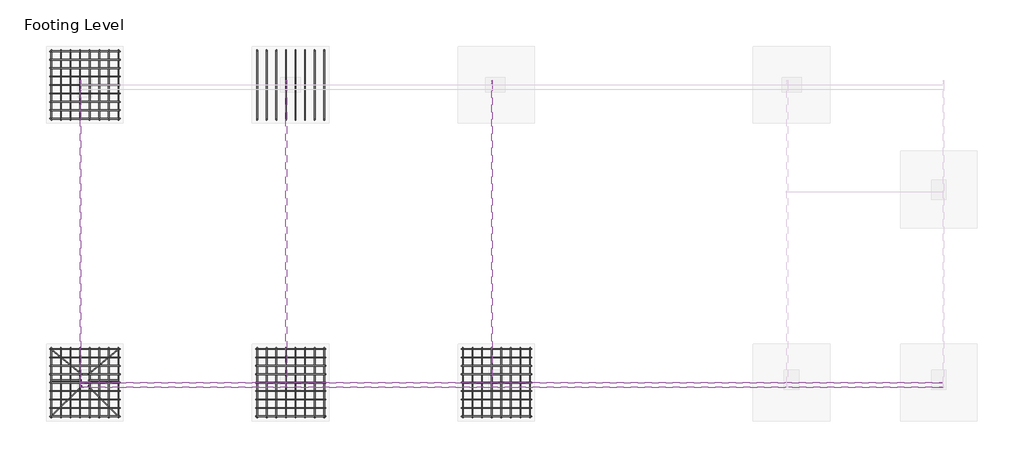
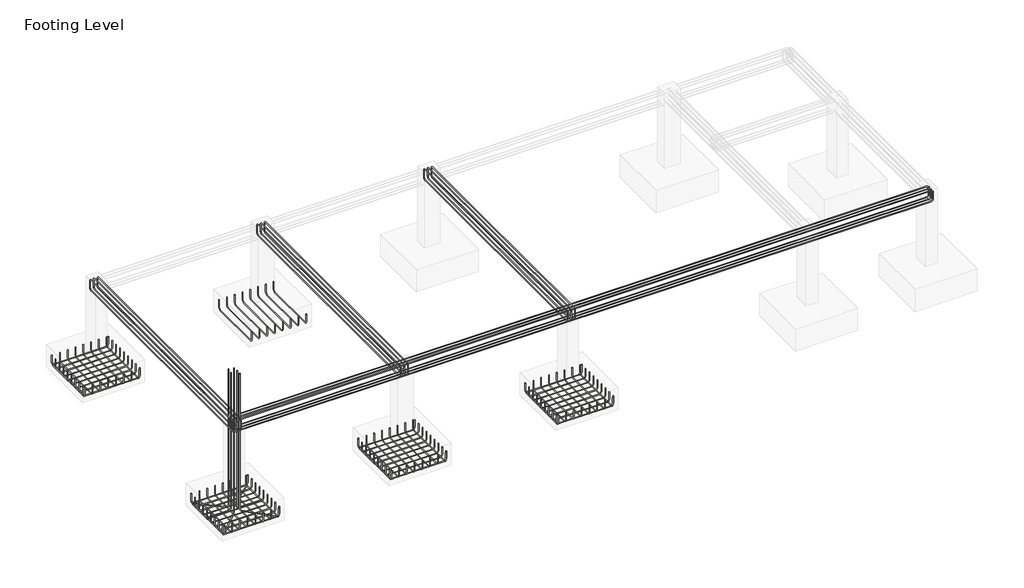
# One storey, part 2 of 3: 23 reinforcing bars.
"""IFC4 building model written with IfcOpenShell, lengths in millimetres."""

from ifc_helpers import new_model, si_unit, point, frame, origin, place, context, project, spatial, polyline, circle_curve, trimmed, segment, composite_curve, source, transform, mapped, element, save
from ifc_brep_helpers import swept_disk

model = new_model("IFC4")

# Units and contexts
model_context = context("Model", 3, world=origin())
ifc_project = project(units=[si_unit("LENGTHUNIT", "METRE", prefix="MILLI")], contexts=[model_context])

# Site, building, storey
site = spatial("IfcSite", under=ifc_project)
building = spatial("IfcBuilding", under=site)
storey = spatial("IfcBuildingStorey", under=building, Name="Footing Level", Elevation=-1524.0)

# Reinforcing bars
placement = place(None, origin())
reinforcing_bar_shape = source(origin(), model_context, "Body", "SolidModel", [
    swept_disk(composite_curve([segment(polyline([(-8741.5465807, -243.2665369, -1724.0), (-8741.5465807, -243.2665369, -1872.0)]), True, "CONTINUOUS"), segment(trimmed(circle_curve(frame((-8741.5465807, -197.2665369, -1872.0), z_axis=(1.0, 0.0, 0.0), x_axis=(0.0, -46.0, 0.0)), 46.0), [point((-8741.5465807, -243.2665369, -1872.0))], [point((-8741.5465807, -197.2665369, -1918.0))], True, "CARTESIAN"), True, "CONTINUOUS"), segment(polyline([(-8741.5465807, -197.2665369, -1918.0), (-8741.5465807, 798.7334631, -1918.0)]), True, "CONTINUOUS"), segment(trimmed(circle_curve(frame((-8741.5465807, 798.7334631, -1872.0), z_axis=(1.0, 0.0, 0.0), x_axis=(0.0, 0.0, -46.0)), 46.0), [point((-8741.5465807, 798.7334631, -1918.0))], [point((-8741.5465807, 844.7334631, -1872.0))], True, "CARTESIAN"), True, "CONTINUOUS"), segment(polyline([(-8741.5465807, 844.7334631, -1872.0), (-8741.5465807, 844.7334631, -1724.0)]), True, "CONTINUOUS")], self_intersect=False), 6.0),
])
element("IfcReinforcingBar", 1, at=placement, inside=storey, context=model_context, shape_type="MappedRepresentation", body=[
    mapped(reinforcing_bar_shape, transform((0.0, 0.0, 0.0), x_axis=(1.0, 0.0, 0.0), y_axis=(0.0, 1.0, 0.0), z_axis=(0.0, 0.0, 1.0))),
    mapped(reinforcing_bar_shape, transform((-149.7374868, 0.0, 0.0), x_axis=(1.0, 0.0, 0.0), y_axis=(0.0, 1.0, 0.0), z_axis=(0.0, 0.0, 1.0))),
    mapped(reinforcing_bar_shape, transform((-299.4749737, 0.0, 0.0), x_axis=(1.0, 0.0, 0.0), y_axis=(0.0, 1.0, 0.0), z_axis=(0.0, 0.0, 1.0))),
    mapped(reinforcing_bar_shape, transform((-449.2124605, 0.0, 0.0), x_axis=(1.0, 0.0, 0.0), y_axis=(0.0, 1.0, 0.0), z_axis=(0.0, 0.0, 1.0))),
    mapped(reinforcing_bar_shape, transform((-598.9499474, 0.0, 0.0), x_axis=(1.0, 0.0, 0.0), y_axis=(0.0, 1.0, 0.0), z_axis=(0.0, 0.0, 1.0))),
    mapped(reinforcing_bar_shape, transform((-748.6874342, 0.0, 0.0), x_axis=(1.0, 0.0, 0.0), y_axis=(0.0, 1.0, 0.0), z_axis=(0.0, 0.0, 1.0))),
    mapped(reinforcing_bar_shape, transform((-898.424921, 0.0, 0.0), x_axis=(1.0, 0.0, 0.0), y_axis=(0.0, 1.0, 0.0), z_axis=(0.0, 0.0, 1.0))),
    mapped(reinforcing_bar_shape, transform((-1048.1624079, 0.0, 0.0), x_axis=(1.0, 0.0, 0.0), y_axis=(0.0, 1.0, 0.0), z_axis=(0.0, 0.0, 1.0))),
])
reinforcing_bar_2_shape = source(origin(), model_context, "Body", "SolidModel", [
    swept_disk(composite_curve([segment(polyline([(-9808.6117524, -224.7796689, -1711.15), (-9808.6117524, -224.7796689, -1859.15)]), True, "CONTINUOUS"), segment(trimmed(circle_curve(frame((-9762.6117524, -224.7796689, -1859.15), z_axis=(0.0, -1.0, 0.0), x_axis=(-46.0, 0.0, 0.0)), 46.0), [point((-9808.6117524, -224.7796689, -1859.15))], [point((-9762.6117524, -224.7796689, -1905.15))], True, "CARTESIAN"), True, "CONTINUOUS"), segment(polyline([(-9762.6117524, -224.7796689, -1905.15), (-8766.6117524, -224.7796689, -1905.15)]), True, "CONTINUOUS"), segment(trimmed(circle_curve(frame((-8766.6117524, -224.7796689, -1859.15), z_axis=(0.0, -1.0, 0.0), x_axis=(0.0, 0.0, -46.0)), 46.0), [point((-8766.6117524, -224.7796689, -1905.15))], [point((-8720.6117524, -224.7796689, -1859.15))], True, "CARTESIAN"), True, "CONTINUOUS"), segment(polyline([(-8720.6117524, -224.7796689, -1859.15), (-8720.6117524, -224.7796689, -1711.15)]), True, "CONTINUOUS")], self_intersect=False), 6.0),
])
element("IfcReinforcingBar", 2, at=placement, inside=storey, context=model_context, shape_type="MappedRepresentation", body=[
    mapped(reinforcing_bar_2_shape, transform((0.0, 0.0, 0.0), x_axis=(1.0, 0.0, 0.0), y_axis=(0.0, 1.0, 0.0), z_axis=(0.0, 0.0, 1.0))),
    mapped(reinforcing_bar_2_shape, transform((0.0, 131.3537501, 0.0), x_axis=(1.0, 0.0, 0.0), y_axis=(0.0, 1.0, 0.0), z_axis=(0.0, 0.0, 1.0))),
    mapped(reinforcing_bar_2_shape, transform((0.0, 262.7075003, 0.0), x_axis=(1.0, 0.0, 0.0), y_axis=(0.0, 1.0, 0.0), z_axis=(0.0, 0.0, 1.0))),
    mapped(reinforcing_bar_2_shape, transform((0.0, 394.0612504, 0.0), x_axis=(1.0, 0.0, 0.0), y_axis=(0.0, 1.0, 0.0), z_axis=(0.0, 0.0, 1.0))),
    mapped(reinforcing_bar_2_shape, transform((0.0, 525.4150006, 0.0), x_axis=(1.0, 0.0, 0.0), y_axis=(0.0, 1.0, 0.0), z_axis=(0.0, 0.0, 1.0))),
    mapped(reinforcing_bar_2_shape, transform((0.0, 656.7687507, 0.0), x_axis=(1.0, 0.0, 0.0), y_axis=(0.0, 1.0, 0.0), z_axis=(0.0, 0.0, 1.0))),
    mapped(reinforcing_bar_2_shape, transform((0.0, 788.1225008, 0.0), x_axis=(1.0, 0.0, 0.0), y_axis=(0.0, 1.0, 0.0), z_axis=(0.0, 0.0, 1.0))),
    mapped(reinforcing_bar_2_shape, transform((0.0, 919.476251, 0.0), x_axis=(1.0, 0.0, 0.0), y_axis=(0.0, 1.0, 0.0), z_axis=(0.0, 0.0, 1.0))),
    mapped(reinforcing_bar_2_shape, transform((0.0, 1050.8300011, 0.0), x_axis=(1.0, 0.0, 0.0), y_axis=(0.0, 1.0, 0.0), z_axis=(0.0, 0.0, 1.0))),
])
reinforcing_bar_3_shape = source(origin(), model_context, "Body", "SolidModel", [
    swept_disk(composite_curve([segment(polyline([(-5528.4465807, -243.2665369, -1724.0), (-5528.4465807, -243.2665369, -1872.0)]), True, "CONTINUOUS"), segment(trimmed(circle_curve(frame((-5528.4465807, -197.2665369, -1872.0), z_axis=(1.0, 0.0, 0.0), x_axis=(0.0, -46.0, 0.0)), 46.0), [point((-5528.4465807, -243.2665369, -1872.0))], [point((-5528.4465807, -197.2665369, -1918.0))], True, "CARTESIAN"), True, "CONTINUOUS"), segment(polyline([(-5528.4465807, -197.2665369, -1918.0), (-5528.4465807, 798.7334631, -1918.0)]), True, "CONTINUOUS"), segment(trimmed(circle_curve(frame((-5528.4465807, 798.7334631, -1872.0), z_axis=(1.0, 0.0, 0.0), x_axis=(0.0, 0.0, -46.0)), 46.0), [point((-5528.4465807, 798.7334631, -1918.0))], [point((-5528.4465807, 844.7334631, -1872.0))], True, "CARTESIAN"), True, "CONTINUOUS"), segment(polyline([(-5528.4465807, 844.7334631, -1872.0), (-5528.4465807, 844.7334631, -1724.0)]), True, "CONTINUOUS")], self_intersect=False), 6.0),
])
element("IfcReinforcingBar", 3, at=placement, inside=storey, context=model_context, shape_type="MappedRepresentation", body=[
    mapped(reinforcing_bar_3_shape, transform((0.0, 0.0, 0.0), x_axis=(1.0, 0.0, 0.0), y_axis=(0.0, 1.0, 0.0), z_axis=(0.0, 0.0, 1.0))),
    mapped(reinforcing_bar_3_shape, transform((-149.7374868, 0.0, 0.0), x_axis=(1.0, 0.0, 0.0), y_axis=(0.0, 1.0, 0.0), z_axis=(0.0, 0.0, 1.0))),
    mapped(reinforcing_bar_3_shape, transform((-299.4749737, 0.0, 0.0), x_axis=(1.0, 0.0, 0.0), y_axis=(0.0, 1.0, 0.0), z_axis=(0.0, 0.0, 1.0))),
    mapped(reinforcing_bar_3_shape, transform((-449.2124605, 0.0, 0.0), x_axis=(1.0, 0.0, 0.0), y_axis=(0.0, 1.0, 0.0), z_axis=(0.0, 0.0, 1.0))),
    mapped(reinforcing_bar_3_shape, transform((-598.9499474, 0.0, 0.0), x_axis=(1.0, 0.0, 0.0), y_axis=(0.0, 1.0, 0.0), z_axis=(0.0, 0.0, 1.0))),
    mapped(reinforcing_bar_3_shape, transform((-748.6874342, 0.0, 0.0), x_axis=(1.0, 0.0, 0.0), y_axis=(0.0, 1.0, 0.0), z_axis=(0.0, 0.0, 1.0))),
    mapped(reinforcing_bar_3_shape, transform((-898.424921, 0.0, 0.0), x_axis=(1.0, 0.0, 0.0), y_axis=(0.0, 1.0, 0.0), z_axis=(0.0, 0.0, 1.0))),
    mapped(reinforcing_bar_3_shape, transform((-1048.1624079, 0.0, 0.0), x_axis=(1.0, 0.0, 0.0), y_axis=(0.0, 1.0, 0.0), z_axis=(0.0, 0.0, 1.0))),
])
reinforcing_bar_4_shape = source(origin(), model_context, "Body", "SolidModel", [
    swept_disk(composite_curve([segment(polyline([(-6595.5117524, -224.7796689, -1711.15), (-6595.5117524, -224.7796689, -1859.15)]), True, "CONTINUOUS"), segment(trimmed(circle_curve(frame((-6549.5117524, -224.7796689, -1859.15), z_axis=(0.0, -1.0, 0.0), x_axis=(-46.0, 0.0, 0.0)), 46.0), [point((-6595.5117524, -224.7796689, -1859.15))], [point((-6549.5117524, -224.7796689, -1905.15))], True, "CARTESIAN"), True, "CONTINUOUS"), segment(polyline([(-6549.5117524, -224.7796689, -1905.15), (-5553.5117524, -224.7796689, -1905.15)]), True, "CONTINUOUS"), segment(trimmed(circle_curve(frame((-5553.5117524, -224.7796689, -1859.15), z_axis=(0.0, -1.0, 0.0), x_axis=(0.0, 0.0, -46.0)), 46.0), [point((-5553.5117524, -224.7796689, -1905.15))], [point((-5507.5117524, -224.7796689, -1859.15))], True, "CARTESIAN"), True, "CONTINUOUS"), segment(polyline([(-5507.5117524, -224.7796689, -1859.15), (-5507.5117524, -224.7796689, -1711.15)]), True, "CONTINUOUS")], self_intersect=False), 6.0),
])
element("IfcReinforcingBar", 4, at=placement, inside=storey, context=model_context, shape_type="MappedRepresentation", body=[
    mapped(reinforcing_bar_4_shape, transform((0.0, 0.0, 0.0), x_axis=(1.0, 0.0, 0.0), y_axis=(0.0, 1.0, 0.0), z_axis=(0.0, 0.0, 1.0))),
    mapped(reinforcing_bar_4_shape, transform((0.0, 131.3537501, 0.0), x_axis=(1.0, 0.0, 0.0), y_axis=(0.0, 1.0, 0.0), z_axis=(0.0, 0.0, 1.0))),
    mapped(reinforcing_bar_4_shape, transform((0.0, 262.7075003, 0.0), x_axis=(1.0, 0.0, 0.0), y_axis=(0.0, 1.0, 0.0), z_axis=(0.0, 0.0, 1.0))),
    mapped(reinforcing_bar_4_shape, transform((0.0, 394.0612504, 0.0), x_axis=(1.0, 0.0, 0.0), y_axis=(0.0, 1.0, 0.0), z_axis=(0.0, 0.0, 1.0))),
    mapped(reinforcing_bar_4_shape, transform((0.0, 525.4150006, 0.0), x_axis=(1.0, 0.0, 0.0), y_axis=(0.0, 1.0, 0.0), z_axis=(0.0, 0.0, 1.0))),
    mapped(reinforcing_bar_4_shape, transform((0.0, 656.7687507, 0.0), x_axis=(1.0, 0.0, 0.0), y_axis=(0.0, 1.0, 0.0), z_axis=(0.0, 0.0, 1.0))),
    mapped(reinforcing_bar_4_shape, transform((0.0, 788.1225008, 0.0), x_axis=(1.0, 0.0, 0.0), y_axis=(0.0, 1.0, 0.0), z_axis=(0.0, 0.0, 1.0))),
    mapped(reinforcing_bar_4_shape, transform((0.0, 919.476251, 0.0), x_axis=(1.0, 0.0, 0.0), y_axis=(0.0, 1.0, 0.0), z_axis=(0.0, 0.0, 1.0))),
    mapped(reinforcing_bar_4_shape, transform((0.0, 1050.8300011, 0.0), x_axis=(1.0, 0.0, 0.0), y_axis=(0.0, 1.0, 0.0), z_axis=(0.0, 0.0, 1.0))),
])
reinforcing_bar_5_shape = source(origin(), model_context, "Body", "SolidModel", [
    swept_disk(composite_curve([segment(polyline([(-2315.3465807, -243.2665369, -1724.0), (-2315.3465807, -243.2665369, -1872.0)]), True, "CONTINUOUS"), segment(trimmed(circle_curve(frame((-2315.3465807, -197.2665369, -1872.0), z_axis=(1.0, 0.0, 0.0), x_axis=(0.0, -46.0, 0.0)), 46.0), [point((-2315.3465807, -243.2665369, -1872.0))], [point((-2315.3465807, -197.2665369, -1918.0))], True, "CARTESIAN"), True, "CONTINUOUS"), segment(polyline([(-2315.3465807, -197.2665369, -1918.0), (-2315.3465807, 798.7334631, -1918.0)]), True, "CONTINUOUS"), segment(trimmed(circle_curve(frame((-2315.3465807, 798.7334631, -1872.0), z_axis=(1.0, 0.0, 0.0), x_axis=(0.0, 0.0, -46.0)), 46.0), [point((-2315.3465807, 798.7334631, -1918.0))], [point((-2315.3465807, 844.7334631, -1872.0))], True, "CARTESIAN"), True, "CONTINUOUS"), segment(polyline([(-2315.3465807, 844.7334631, -1872.0), (-2315.3465807, 844.7334631, -1724.0)]), True, "CONTINUOUS")], self_intersect=False), 6.0),
])
element("IfcReinforcingBar", 5, at=placement, inside=storey, context=model_context, shape_type="MappedRepresentation", body=[
    mapped(reinforcing_bar_5_shape, transform((0.0, 0.0, 0.0), x_axis=(1.0, 0.0, 0.0), y_axis=(0.0, 1.0, 0.0), z_axis=(0.0, 0.0, 1.0))),
    mapped(reinforcing_bar_5_shape, transform((-149.7374868, 0.0, 0.0), x_axis=(1.0, 0.0, 0.0), y_axis=(0.0, 1.0, 0.0), z_axis=(0.0, 0.0, 1.0))),
    mapped(reinforcing_bar_5_shape, transform((-299.4749737, 0.0, 0.0), x_axis=(1.0, 0.0, 0.0), y_axis=(0.0, 1.0, 0.0), z_axis=(0.0, 0.0, 1.0))),
    mapped(reinforcing_bar_5_shape, transform((-449.2124605, 0.0, 0.0), x_axis=(1.0, 0.0, 0.0), y_axis=(0.0, 1.0, 0.0), z_axis=(0.0, 0.0, 1.0))),
    mapped(reinforcing_bar_5_shape, transform((-598.9499474, 0.0, 0.0), x_axis=(1.0, 0.0, 0.0), y_axis=(0.0, 1.0, 0.0), z_axis=(0.0, 0.0, 1.0))),
    mapped(reinforcing_bar_5_shape, transform((-748.6874342, 0.0, 0.0), x_axis=(1.0, 0.0, 0.0), y_axis=(0.0, 1.0, 0.0), z_axis=(0.0, 0.0, 1.0))),
    mapped(reinforcing_bar_5_shape, transform((-898.424921, 0.0, 0.0), x_axis=(1.0, 0.0, 0.0), y_axis=(0.0, 1.0, 0.0), z_axis=(0.0, 0.0, 1.0))),
    mapped(reinforcing_bar_5_shape, transform((-1048.1624079, 0.0, 0.0), x_axis=(1.0, 0.0, 0.0), y_axis=(0.0, 1.0, 0.0), z_axis=(0.0, 0.0, 1.0))),
])
reinforcing_bar_6_shape = source(origin(), model_context, "Body", "SolidModel", [
    swept_disk(composite_curve([segment(polyline([(-3382.4117524, -224.7796689, -1711.15), (-3382.4117524, -224.7796689, -1859.15)]), True, "CONTINUOUS"), segment(trimmed(circle_curve(frame((-3336.4117524, -224.7796689, -1859.15), z_axis=(0.0, -1.0, 0.0), x_axis=(-46.0, 0.0, 0.0)), 46.0), [point((-3382.4117524, -224.7796689, -1859.15))], [point((-3336.4117524, -224.7796689, -1905.15))], True, "CARTESIAN"), True, "CONTINUOUS"), segment(polyline([(-3336.4117524, -224.7796689, -1905.15), (-2340.4117524, -224.7796689, -1905.15)]), True, "CONTINUOUS"), segment(trimmed(circle_curve(frame((-2340.4117524, -224.7796689, -1859.15), z_axis=(0.0, -1.0, 0.0), x_axis=(0.0, 0.0, -46.0)), 46.0), [point((-2340.4117524, -224.7796689, -1905.15))], [point((-2294.4117524, -224.7796689, -1859.15))], True, "CARTESIAN"), True, "CONTINUOUS"), segment(polyline([(-2294.4117524, -224.7796689, -1859.15), (-2294.4117524, -224.7796689, -1711.15)]), True, "CONTINUOUS")], self_intersect=False), 6.0),
])
element("IfcReinforcingBar", 6, at=placement, inside=storey, context=model_context, shape_type="MappedRepresentation", body=[
    mapped(reinforcing_bar_6_shape, transform((0.0, 0.0, 0.0), x_axis=(1.0, 0.0, 0.0), y_axis=(0.0, 1.0, 0.0), z_axis=(0.0, 0.0, 1.0))),
    mapped(reinforcing_bar_6_shape, transform((0.0, 131.3537501, 0.0), x_axis=(1.0, 0.0, 0.0), y_axis=(0.0, 1.0, 0.0), z_axis=(0.0, 0.0, 1.0))),
    mapped(reinforcing_bar_6_shape, transform((0.0, 262.7075003, 0.0), x_axis=(1.0, 0.0, 0.0), y_axis=(0.0, 1.0, 0.0), z_axis=(0.0, 0.0, 1.0))),
    mapped(reinforcing_bar_6_shape, transform((0.0, 394.0612504, 0.0), x_axis=(1.0, 0.0, 0.0), y_axis=(0.0, 1.0, 0.0), z_axis=(0.0, 0.0, 1.0))),
    mapped(reinforcing_bar_6_shape, transform((0.0, 525.4150006, 0.0), x_axis=(1.0, 0.0, 0.0), y_axis=(0.0, 1.0, 0.0), z_axis=(0.0, 0.0, 1.0))),
    mapped(reinforcing_bar_6_shape, transform((0.0, 656.7687507, 0.0), x_axis=(1.0, 0.0, 0.0), y_axis=(0.0, 1.0, 0.0), z_axis=(0.0, 0.0, 1.0))),
    mapped(reinforcing_bar_6_shape, transform((0.0, 788.1225008, 0.0), x_axis=(1.0, 0.0, 0.0), y_axis=(0.0, 1.0, 0.0), z_axis=(0.0, 0.0, 1.0))),
    mapped(reinforcing_bar_6_shape, transform((0.0, 919.476251, 0.0), x_axis=(1.0, 0.0, 0.0), y_axis=(0.0, 1.0, 0.0), z_axis=(0.0, 0.0, 1.0))),
    mapped(reinforcing_bar_6_shape, transform((0.0, 1050.8300011, 0.0), x_axis=(1.0, 0.0, 0.0), y_axis=(0.0, 1.0, 0.0), z_axis=(0.0, 0.0, 1.0))),
])
reinforcing_bar_7_shape = source(origin(), model_context, "Body", "SolidModel", [
    swept_disk(composite_curve([segment(polyline([(-5528.4465807, 4404.9334631, -1724.0), (-5528.4465807, 4404.9334631, -1872.0)]), True, "CONTINUOUS"), segment(trimmed(circle_curve(frame((-5528.4465807, 4450.9334631, -1872.0), z_axis=(1.0, 0.0, 0.0), x_axis=(0.0, -46.0, 0.0)), 46.0), [point((-5528.4465807, 4404.9334631, -1872.0))], [point((-5528.4465807, 4450.9334631, -1918.0))], True, "CARTESIAN"), True, "CONTINUOUS"), segment(polyline([(-5528.4465807, 4450.9334631, -1918.0), (-5528.4465807, 5446.9334631, -1918.0)]), True, "CONTINUOUS"), segment(trimmed(circle_curve(frame((-5528.4465807, 5446.9334631, -1872.0), z_axis=(1.0, 0.0, 0.0), x_axis=(0.0, 0.0, -46.0)), 46.0), [point((-5528.4465807, 5446.9334631, -1918.0))], [point((-5528.4465807, 5492.9334631, -1872.0))], True, "CARTESIAN"), True, "CONTINUOUS"), segment(polyline([(-5528.4465807, 5492.9334631, -1872.0), (-5528.4465807, 5492.9334631, -1724.0)]), True, "CONTINUOUS")], self_intersect=False), 6.0),
])
element("IfcReinforcingBar", 7, at=placement, inside=storey, context=model_context, shape_type="MappedRepresentation", body=[
    mapped(reinforcing_bar_7_shape, transform((0.0, 0.0, 0.0), x_axis=(1.0, 0.0, 0.0), y_axis=(0.0, 1.0, 0.0), z_axis=(0.0, 0.0, 1.0))),
    mapped(reinforcing_bar_7_shape, transform((-149.7374868, 0.0, 0.0), x_axis=(1.0, 0.0, 0.0), y_axis=(0.0, 1.0, 0.0), z_axis=(0.0, 0.0, 1.0))),
    mapped(reinforcing_bar_7_shape, transform((-299.4749737, 0.0, 0.0), x_axis=(1.0, 0.0, 0.0), y_axis=(0.0, 1.0, 0.0), z_axis=(0.0, 0.0, 1.0))),
    mapped(reinforcing_bar_7_shape, transform((-449.2124605, 0.0, 0.0), x_axis=(1.0, 0.0, 0.0), y_axis=(0.0, 1.0, 0.0), z_axis=(0.0, 0.0, 1.0))),
    mapped(reinforcing_bar_7_shape, transform((-598.9499474, 0.0, 0.0), x_axis=(1.0, 0.0, 0.0), y_axis=(0.0, 1.0, 0.0), z_axis=(0.0, 0.0, 1.0))),
    mapped(reinforcing_bar_7_shape, transform((-748.6874342, 0.0, 0.0), x_axis=(1.0, 0.0, 0.0), y_axis=(0.0, 1.0, 0.0), z_axis=(0.0, 0.0, 1.0))),
    mapped(reinforcing_bar_7_shape, transform((-898.424921, 0.0, 0.0), x_axis=(1.0, 0.0, 0.0), y_axis=(0.0, 1.0, 0.0), z_axis=(0.0, 0.0, 1.0))),
    mapped(reinforcing_bar_7_shape, transform((-1048.1624079, 0.0, 0.0), x_axis=(1.0, 0.0, 0.0), y_axis=(0.0, 1.0, 0.0), z_axis=(0.0, 0.0, 1.0))),
])
reinforcing_bar_8_shape = source(origin(), model_context, "Body", "SolidModel", [
    swept_disk(composite_curve([segment(polyline([(-8741.5465807, 4404.9334631, -1724.0), (-8741.5465807, 4404.9334631, -1872.0)]), True, "CONTINUOUS"), segment(trimmed(circle_curve(frame((-8741.5465807, 4450.9334631, -1872.0), z_axis=(1.0, 0.0, 0.0), x_axis=(0.0, -46.0, 0.0)), 46.0), [point((-8741.5465807, 4404.9334631, -1872.0))], [point((-8741.5465807, 4450.9334631, -1918.0))], True, "CARTESIAN"), True, "CONTINUOUS"), segment(polyline([(-8741.5465807, 4450.9334631, -1918.0), (-8741.5465807, 5446.9334631, -1918.0)]), True, "CONTINUOUS"), segment(trimmed(circle_curve(frame((-8741.5465807, 5446.9334631, -1872.0), z_axis=(1.0, 0.0, 0.0), x_axis=(0.0, 0.0, -46.0)), 46.0), [point((-8741.5465807, 5446.9334631, -1918.0))], [point((-8741.5465807, 5492.9334631, -1872.0))], True, "CARTESIAN"), True, "CONTINUOUS"), segment(polyline([(-8741.5465807, 5492.9334631, -1872.0), (-8741.5465807, 5492.9334631, -1724.0)]), True, "CONTINUOUS")], self_intersect=False), 6.0),
])
element("IfcReinforcingBar", 8, at=placement, inside=storey, context=model_context, shape_type="MappedRepresentation", body=[
    mapped(reinforcing_bar_8_shape, transform((0.0, 0.0, 0.0), x_axis=(1.0, 0.0, 0.0), y_axis=(0.0, 1.0, 0.0), z_axis=(0.0, 0.0, 1.0))),
    mapped(reinforcing_bar_8_shape, transform((-149.7374868, 0.0, 0.0), x_axis=(1.0, 0.0, 0.0), y_axis=(0.0, 1.0, 0.0), z_axis=(0.0, 0.0, 1.0))),
    mapped(reinforcing_bar_8_shape, transform((-299.4749737, 0.0, 0.0), x_axis=(1.0, 0.0, 0.0), y_axis=(0.0, 1.0, 0.0), z_axis=(0.0, 0.0, 1.0))),
    mapped(reinforcing_bar_8_shape, transform((-449.2124605, 0.0, 0.0), x_axis=(1.0, 0.0, 0.0), y_axis=(0.0, 1.0, 0.0), z_axis=(0.0, 0.0, 1.0))),
    mapped(reinforcing_bar_8_shape, transform((-598.9499474, 0.0, 0.0), x_axis=(1.0, 0.0, 0.0), y_axis=(0.0, 1.0, 0.0), z_axis=(0.0, 0.0, 1.0))),
    mapped(reinforcing_bar_8_shape, transform((-748.6874342, 0.0, 0.0), x_axis=(1.0, 0.0, 0.0), y_axis=(0.0, 1.0, 0.0), z_axis=(0.0, 0.0, 1.0))),
    mapped(reinforcing_bar_8_shape, transform((-898.424921, 0.0, 0.0), x_axis=(1.0, 0.0, 0.0), y_axis=(0.0, 1.0, 0.0), z_axis=(0.0, 0.0, 1.0))),
    mapped(reinforcing_bar_8_shape, transform((-1048.1624079, 0.0, 0.0), x_axis=(1.0, 0.0, 0.0), y_axis=(0.0, 1.0, 0.0), z_axis=(0.0, 0.0, 1.0))),
])
reinforcing_bar_9_shape = source(origin(), model_context, "Body", "SolidModel", [
    swept_disk(composite_curve([segment(polyline([(-9808.6117524, 4423.4203311, -1711.15), (-9808.6117524, 4423.4203311, -1859.15)]), True, "CONTINUOUS"), segment(trimmed(circle_curve(frame((-9762.6117524, 4423.4203311, -1859.15), z_axis=(0.0, -1.0, 0.0), x_axis=(-46.0, 0.0, 0.0)), 46.0), [point((-9808.6117524, 4423.4203311, -1859.15))], [point((-9762.6117524, 4423.4203311, -1905.15))], True, "CARTESIAN"), True, "CONTINUOUS"), segment(polyline([(-9762.6117524, 4423.4203311, -1905.15), (-8766.6117524, 4423.4203311, -1905.15)]), True, "CONTINUOUS"), segment(trimmed(circle_curve(frame((-8766.6117524, 4423.4203311, -1859.15), z_axis=(0.0, -1.0, 0.0), x_axis=(0.0, 0.0, -46.0)), 46.0), [point((-8766.6117524, 4423.4203311, -1905.15))], [point((-8720.6117524, 4423.4203311, -1859.15))], True, "CARTESIAN"), True, "CONTINUOUS"), segment(polyline([(-8720.6117524, 4423.4203311, -1859.15), (-8720.6117524, 4423.4203311, -1711.15)]), True, "CONTINUOUS")], self_intersect=False), 6.0),
])
element("IfcReinforcingBar", 9, at=placement, inside=storey, context=model_context, shape_type="MappedRepresentation", body=[
    mapped(reinforcing_bar_9_shape, transform((0.0, 0.0, 0.0), x_axis=(1.0, 0.0, 0.0), y_axis=(0.0, 1.0, 0.0), z_axis=(0.0, 0.0, 1.0))),
    mapped(reinforcing_bar_9_shape, transform((0.0, 131.3537501, 0.0), x_axis=(1.0, 0.0, 0.0), y_axis=(0.0, 1.0, 0.0), z_axis=(0.0, 0.0, 1.0))),
    mapped(reinforcing_bar_9_shape, transform((0.0, 262.7075003, 0.0), x_axis=(1.0, 0.0, 0.0), y_axis=(0.0, 1.0, 0.0), z_axis=(0.0, 0.0, 1.0))),
    mapped(reinforcing_bar_9_shape, transform((0.0, 394.0612504, 0.0), x_axis=(1.0, 0.0, 0.0), y_axis=(0.0, 1.0, 0.0), z_axis=(0.0, 0.0, 1.0))),
    mapped(reinforcing_bar_9_shape, transform((0.0, 525.4150006, 0.0), x_axis=(1.0, 0.0, 0.0), y_axis=(0.0, 1.0, 0.0), z_axis=(0.0, 0.0, 1.0))),
    mapped(reinforcing_bar_9_shape, transform((0.0, 656.7687507, 0.0), x_axis=(1.0, 0.0, 0.0), y_axis=(0.0, 1.0, 0.0), z_axis=(0.0, 0.0, 1.0))),
    mapped(reinforcing_bar_9_shape, transform((0.0, 788.1225008, 0.0), x_axis=(1.0, 0.0, 0.0), y_axis=(0.0, 1.0, 0.0), z_axis=(0.0, 0.0, 1.0))),
    mapped(reinforcing_bar_9_shape, transform((0.0, 919.476251, 0.0), x_axis=(1.0, 0.0, 0.0), y_axis=(0.0, 1.0, 0.0), z_axis=(0.0, 0.0, 1.0))),
    mapped(reinforcing_bar_9_shape, transform((0.0, 1050.8300011, 0.0), x_axis=(1.0, 0.0, 0.0), y_axis=(0.0, 1.0, 0.0), z_axis=(0.0, 0.0, 1.0))),
])
element("IfcReinforcingBar", 10, at=placement, inside=storey, context=model_context, shape_type="SolidModel", body=[
    swept_disk(composite_curve([segment(polyline([(-9209.9729913, 244.7072019, 877.2694454), (-9209.9729913, 244.7072019, -1868.0)]), True, "CONTINUOUS"), segment(trimmed(circle_curve(frame((-9177.4460793, 212.1802899, -1868.0), z_axis=(-0.7071067811865491, -0.707106781186546, 0.0), x_axis=(-32.526911999999356, 32.52691200000001, 0.0)), 46.0), [point((-9209.9729913, 244.7072019, -1868.0))], [point((-9177.4460793, 212.1802899, -1914.0))], True, "CARTESIAN"), True, "CONTINUOUS"), segment(polyline([(-9177.4460793, 212.1802899, -1914.0), (-8771.7428199, -193.5229695, -1914.0)]), True, "CONTINUOUS")], self_intersect=False), 6.0),
])
element("IfcReinforcingBar", 11, at=placement, inside=storey, context=model_context, shape_type="SolidModel", body=[
    swept_disk(composite_curve([segment(polyline([(-9318.7998971, 245.6611074, 884.8983833), (-9318.7998971, 245.6611074, -1868.0)]), True, "CONTINUOUS"), segment(trimmed(circle_curve(frame((-9351.326809, 213.1341954, -1868.0), z_axis=(-0.7071067811865491, 0.707106781186546, 0.0), x_axis=(32.526911900000414, 32.52691199999998, 0.0)), 46.0), [point((-9318.7998971, 245.6611074, -1868.0))], [point((-9351.326809, 213.1341954, -1914.0))], True, "CARTESIAN"), True, "CONTINUOUS"), segment(polyline([(-9351.326809, 213.1341954, -1914.0), (-9763.4563428, -198.9953384, -1914.0)]), True, "CONTINUOUS")], self_intersect=False), 6.0),
])
element("IfcReinforcingBar", 12, at=placement, inside=storey, context=model_context, shape_type="SolidModel", body=[
    swept_disk(composite_curve([segment(polyline([(-9211.2828277, 432.9867911, 871.8711989), (-9211.2828277, 432.9867911, -1868.0)]), True, "CONTINUOUS"), segment(trimmed(circle_curve(frame((-9175.7367573, 462.1839978, -1868.0), z_axis=(0.634721884628903, -0.7727406610067402, 0.0), x_axis=(-35.546070400001554, -29.19720669999998, 0.0)), 46.0), [point((-9211.2828277, 432.9867911, -1868.0))], [point((-9175.7367573, 462.1839978, -1914.0))], True, "CARTESIAN"), True, "CONTINUOUS"), segment(polyline([(-9175.7367573, 462.1839978, -1914.0), (-8753.4008173, 809.0867522, -1914.0)]), True, "CONTINUOUS")], self_intersect=False), 6.0),
])
element("IfcReinforcingBar", 13, at=placement, inside=storey, context=model_context, shape_type="SolidModel", body=[
    swept_disk(composite_curve([segment(polyline([(-9317.9839747, 432.7322479, 890.3940928), (-9317.9839747, 432.7322479, -1868.0)]), True, "CONTINUOUS"), segment(trimmed(circle_curve(frame((-9353.5300451, 461.9294546, -1868.0), z_axis=(0.634721884628903, 0.7727406610067401, 0.0), x_axis=(35.546070399999735, -29.19720669999998, 0.0)), 46.0), [point((-9317.9839747, 432.7322479, -1868.0))], [point((-9353.5300451, 461.9294546, -1914.0))], True, "CARTESIAN"), True, "CONTINUOUS"), segment(polyline([(-9353.5300451, 461.9294546, -1914.0), (-9777.6976875, 810.3367522, -1914.0)]), True, "CONTINUOUS")], self_intersect=False), 6.0),
])
element("IfcReinforcingBar", 14, at=placement, inside=storey, context=model_context, shape_type="SolidModel", body=[
    swept_disk(composite_curve([segment(polyline([(-9204.3117524, 339.6230123, 875.7528218), (-9204.3117524, 339.6230123, -1868.0)]), True, "CONTINUOUS"), segment(trimmed(circle_curve(frame((-9158.3117524, 339.6230123, -1868.0), z_axis=(0.0, -1.0, 0.0), x_axis=(-46.0, 0.0, 0.0)), 46.0), [point((-9204.3117524, 339.6230123, -1868.0))], [point((-9158.3117524, 339.6230123, -1914.0))], True, "CARTESIAN"), True, "CONTINUOUS"), segment(polyline([(-9158.3117524, 339.6230123, -1914.0), (-8747.3359391, 339.6230123, -1914.0)]), True, "CONTINUOUS")], self_intersect=False), 6.0),
])
element("IfcReinforcingBar", 15, at=placement, inside=storey, context=model_context, shape_type="SolidModel", body=[
    swept_disk(composite_curve([segment(polyline([(-9324.9117524, 339.6230123, 879.2840812), (-9324.9117524, 339.6230123, -1868.0)]), True, "CONTINUOUS"), segment(trimmed(circle_curve(frame((-9370.9117524, 339.6230123, -1868.0), z_axis=(0.0, 1.0, 0.0), x_axis=(46.0, 0.0, 0.0)), 46.0), [point((-9324.9117524, 339.6230123, -1868.0))], [point((-9370.9117524, 339.6230123, -1914.0))], True, "CARTESIAN"), True, "CONTINUOUS"), segment(polyline([(-9370.9117524, 339.6230123, -1914.0), (-9784.4222077, 339.6230123, -1914.0)]), True, "CONTINUOUS")], self_intersect=False), 6.0),
])
reinforcing_bar_10_shape = source(origin(), model_context, "Body", "SolidModel", [
    swept_disk(composite_curve([segment(polyline([(-9335.8112474, 5017.2334631, -237.1005051), (-9335.8112474, 5017.2334631, -89.1005051)]), True, "CONTINUOUS"), segment(trimmed(circle_curve(frame((-9335.8112474, 4971.2334631, -89.1005051), z_axis=(1.0, 0.0, 0.0), x_axis=(0.0, 46.0, 0.0)), 46.0), [point((-9335.8112474, 5017.2334631, -89.1005051))], [point((-9335.8112474, 4971.2334631, -43.1005051))], True, "CARTESIAN"), True, "CONTINUOUS"), segment(polyline([(-9335.8112474, 4971.2334631, -43.1005051), (-9335.8112474, 278.4334631, -43.1005051)]), True, "CONTINUOUS"), segment(trimmed(circle_curve(frame((-9335.8112474, 278.4334631, -89.1005051), z_axis=(1.0, 0.0, 0.0), x_axis=(0.0, 0.0, 46.00000000000001)), 46.0), [point((-9335.8112474, 278.4334631, -43.1005051))], [point((-9335.8112474, 232.4334631, -89.1005051))], True, "CARTESIAN"), True, "CONTINUOUS"), segment(polyline([(-9335.8112474, 232.4334631, -89.1005051), (-9335.8112474, 232.4334631, -237.1005051)]), True, "CONTINUOUS")], self_intersect=False), 6.0),
])
element("IfcReinforcingBar", 16, at=placement, inside=storey, context=model_context, shape_type="MappedRepresentation", body=[
    mapped(reinforcing_bar_10_shape, transform((0.0, 0.0, 0.0), x_axis=(1.0, 0.0, 0.0), y_axis=(0.0, 1.0, 0.0), z_axis=(0.0, 0.0, 1.0))),
    mapped(reinforcing_bar_10_shape, transform((71.1994949, 0.0, 0.0), x_axis=(1.0, 0.0, 0.0), y_axis=(0.0, 1.0, 0.0), z_axis=(0.0, 0.0, 1.0))),
    mapped(reinforcing_bar_10_shape, transform((142.3989899, 0.0, 0.0), x_axis=(1.0, 0.0, 0.0), y_axis=(0.0, 1.0, 0.0), z_axis=(0.0, 0.0, 1.0))),
])
reinforcing_bar_11_shape = source(origin(), model_context, "Body", "SolidModel", [
    swept_disk(composite_curve([segment(polyline([(-9335.8112474, 5017.2334631, -67.6994949), (-9335.8112474, 5017.2334631, -215.6994949)]), True, "CONTINUOUS"), segment(trimmed(circle_curve(frame((-9335.8112474, 4971.2334631, -215.6994949), z_axis=(-1.0, 0.0, 0.0), x_axis=(0.0, 46.0, 0.0)), 46.0), [point((-9335.8112474, 5017.2334631, -215.6994949))], [point((-9335.8112474, 4971.2334631, -261.6994949))], True, "CARTESIAN"), True, "CONTINUOUS"), segment(polyline([(-9335.8112474, 4971.2334631, -261.6994949), (-9335.8112474, 278.4334631, -261.6994949)]), True, "CONTINUOUS"), segment(trimmed(circle_curve(frame((-9335.8112474, 278.4334631, -215.6994949), z_axis=(-1.0, 0.0, 0.0), x_axis=(0.0, 0.0, -46.0)), 46.0), [point((-9335.8112474, 278.4334631, -261.6994949))], [point((-9335.8112474, 232.4334631, -215.6994949))], True, "CARTESIAN"), True, "CONTINUOUS"), segment(polyline([(-9335.8112474, 232.4334631, -215.6994949), (-9335.8112474, 232.4334631, -67.6994949)]), True, "CONTINUOUS")], self_intersect=False), 6.0),
])
element("IfcReinforcingBar", 17, at=placement, inside=storey, context=model_context, shape_type="MappedRepresentation", body=[
    mapped(reinforcing_bar_11_shape, transform((0.0, 0.0, 0.0), x_axis=(1.0, 0.0, 0.0), y_axis=(0.0, 1.0, 0.0), z_axis=(0.0, 0.0, 1.0))),
    mapped(reinforcing_bar_11_shape, transform((71.1994949, 0.0, 0.0), x_axis=(1.0, 0.0, 0.0), y_axis=(0.0, 1.0, 0.0), z_axis=(0.0, 0.0, 1.0))),
    mapped(reinforcing_bar_11_shape, transform((142.3989899, 0.0, 0.0), x_axis=(1.0, 0.0, 0.0), y_axis=(0.0, 1.0, 0.0), z_axis=(0.0, 0.0, 1.0))),
])
reinforcing_bar_12_shape = source(origin(), model_context, "Body", "SolidModel", [
    swept_disk(composite_curve([segment(polyline([(-6122.7112474, 5017.2334631, -237.1005051), (-6122.7112474, 5017.2334631, -89.1005051)]), True, "CONTINUOUS"), segment(trimmed(circle_curve(frame((-6122.7112474, 4971.2334631, -89.1005051), z_axis=(1.0, 0.0, 0.0), x_axis=(0.0, 46.0, 0.0)), 46.0), [point((-6122.7112474, 5017.2334631, -89.1005051))], [point((-6122.7112474, 4971.2334631, -43.1005051))], True, "CARTESIAN"), True, "CONTINUOUS"), segment(polyline([(-6122.7112474, 4971.2334631, -43.1005051), (-6122.7112474, 278.4334631, -43.1005051)]), True, "CONTINUOUS"), segment(trimmed(circle_curve(frame((-6122.7112474, 278.4334631, -89.1005051), z_axis=(1.0, 0.0, 0.0), x_axis=(0.0, 0.0, 46.00000000000001)), 46.0), [point((-6122.7112474, 278.4334631, -43.1005051))], [point((-6122.7112474, 232.4334631, -89.1005051))], True, "CARTESIAN"), True, "CONTINUOUS"), segment(polyline([(-6122.7112474, 232.4334631, -89.1005051), (-6122.7112474, 232.4334631, -237.1005051)]), True, "CONTINUOUS")], self_intersect=False), 6.0),
])
element("IfcReinforcingBar", 18, at=placement, inside=storey, context=model_context, shape_type="MappedRepresentation", body=[
    mapped(reinforcing_bar_12_shape, transform((0.0, 0.0, 0.0), x_axis=(1.0, 0.0, 0.0), y_axis=(0.0, 1.0, 0.0), z_axis=(0.0, 0.0, 1.0))),
    mapped(reinforcing_bar_12_shape, transform((71.1994949, 0.0, 0.0), x_axis=(1.0, 0.0, 0.0), y_axis=(0.0, 1.0, 0.0), z_axis=(0.0, 0.0, 1.0))),
    mapped(reinforcing_bar_12_shape, transform((142.3989899, 0.0, 0.0), x_axis=(1.0, 0.0, 0.0), y_axis=(0.0, 1.0, 0.0), z_axis=(0.0, 0.0, 1.0))),
])
reinforcing_bar_13_shape = source(origin(), model_context, "Body", "SolidModel", [
    swept_disk(composite_curve([segment(polyline([(-6122.7112474, 5017.2334631, -67.6994949), (-6122.7112474, 5017.2334631, -215.6994949)]), True, "CONTINUOUS"), segment(trimmed(circle_curve(frame((-6122.7112474, 4971.2334631, -215.6994949), z_axis=(-1.0, 0.0, 0.0), x_axis=(0.0, 46.0, 0.0)), 46.0), [point((-6122.7112474, 5017.2334631, -215.6994949))], [point((-6122.7112474, 4971.2334631, -261.6994949))], True, "CARTESIAN"), True, "CONTINUOUS"), segment(polyline([(-6122.7112474, 4971.2334631, -261.6994949), (-6122.7112474, 278.4334631, -261.6994949)]), True, "CONTINUOUS"), segment(trimmed(circle_curve(frame((-6122.7112474, 278.4334631, -215.6994949), z_axis=(-1.0, 0.0, 0.0), x_axis=(0.0, 0.0, -46.0)), 46.0), [point((-6122.7112474, 278.4334631, -261.6994949))], [point((-6122.7112474, 232.4334631, -215.6994949))], True, "CARTESIAN"), True, "CONTINUOUS"), segment(polyline([(-6122.7112474, 232.4334631, -215.6994949), (-6122.7112474, 232.4334631, -67.6994949)]), True, "CONTINUOUS")], self_intersect=False), 6.0),
])
element("IfcReinforcingBar", 19, at=placement, inside=storey, context=model_context, shape_type="MappedRepresentation", body=[
    mapped(reinforcing_bar_13_shape, transform((0.0, 0.0, 0.0), x_axis=(1.0, 0.0, 0.0), y_axis=(0.0, 1.0, 0.0), z_axis=(0.0, 0.0, 1.0))),
    mapped(reinforcing_bar_13_shape, transform((71.1994949, 0.0, 0.0), x_axis=(1.0, 0.0, 0.0), y_axis=(0.0, 1.0, 0.0), z_axis=(0.0, 0.0, 1.0))),
    mapped(reinforcing_bar_13_shape, transform((142.3989899, 0.0, 0.0), x_axis=(1.0, 0.0, 0.0), y_axis=(0.0, 1.0, 0.0), z_axis=(0.0, 0.0, 1.0))),
])
reinforcing_bar_14_shape = source(origin(), model_context, "Body", "SolidModel", [
    swept_disk(composite_curve([segment(polyline([(-2909.6112474, 5017.2334631, -237.1005051), (-2909.6112474, 5017.2334631, -89.1005051)]), True, "CONTINUOUS"), segment(trimmed(circle_curve(frame((-2909.6112474, 4971.2334631, -89.1005051), z_axis=(1.0, 0.0, 0.0), x_axis=(0.0, 46.0, 0.0)), 46.0), [point((-2909.6112474, 5017.2334631, -89.1005051))], [point((-2909.6112474, 4971.2334631, -43.1005051))], True, "CARTESIAN"), True, "CONTINUOUS"), segment(polyline([(-2909.6112474, 4971.2334631, -43.1005051), (-2909.6112474, 278.4334631, -43.1005051)]), True, "CONTINUOUS"), segment(trimmed(circle_curve(frame((-2909.6112474, 278.4334631, -89.1005051), z_axis=(1.0, 0.0, 0.0), x_axis=(0.0, 0.0, 46.00000000000001)), 46.0), [point((-2909.6112474, 278.4334631, -43.1005051))], [point((-2909.6112474, 232.4334631, -89.1005051))], True, "CARTESIAN"), True, "CONTINUOUS"), segment(polyline([(-2909.6112474, 232.4334631, -89.1005051), (-2909.6112474, 232.4334631, -237.1005051)]), True, "CONTINUOUS")], self_intersect=False), 6.0),
])
element("IfcReinforcingBar", 20, at=placement, inside=storey, context=model_context, shape_type="MappedRepresentation", body=[
    mapped(reinforcing_bar_14_shape, transform((0.0, 0.0, 0.0), x_axis=(1.0, 0.0, 0.0), y_axis=(0.0, 1.0, 0.0), z_axis=(0.0, 0.0, 1.0))),
    mapped(reinforcing_bar_14_shape, transform((71.1994949, 0.0, 0.0), x_axis=(1.0, 0.0, 0.0), y_axis=(0.0, 1.0, 0.0), z_axis=(0.0, 0.0, 1.0))),
    mapped(reinforcing_bar_14_shape, transform((142.3989899, 0.0, 0.0), x_axis=(1.0, 0.0, 0.0), y_axis=(0.0, 1.0, 0.0), z_axis=(0.0, 0.0, 1.0))),
])
reinforcing_bar_15_shape = source(origin(), model_context, "Body", "SolidModel", [
    swept_disk(composite_curve([segment(polyline([(-2909.6112474, 5017.2334631, -67.6994949), (-2909.6112474, 5017.2334631, -215.6994949)]), True, "CONTINUOUS"), segment(trimmed(circle_curve(frame((-2909.6112474, 4971.2334631, -215.6994949), z_axis=(-1.0, 0.0, 0.0), x_axis=(0.0, 46.0, 0.0)), 46.0), [point((-2909.6112474, 5017.2334631, -215.6994949))], [point((-2909.6112474, 4971.2334631, -261.6994949))], True, "CARTESIAN"), True, "CONTINUOUS"), segment(polyline([(-2909.6112474, 4971.2334631, -261.6994949), (-2909.6112474, 278.4334631, -261.6994949)]), True, "CONTINUOUS"), segment(trimmed(circle_curve(frame((-2909.6112474, 278.4334631, -215.6994949), z_axis=(-1.0, 0.0, 0.0), x_axis=(0.0, 0.0, -46.0)), 46.0), [point((-2909.6112474, 278.4334631, -261.6994949))], [point((-2909.6112474, 232.4334631, -215.6994949))], True, "CARTESIAN"), True, "CONTINUOUS"), segment(polyline([(-2909.6112474, 232.4334631, -215.6994949), (-2909.6112474, 232.4334631, -67.6994949)]), True, "CONTINUOUS")], self_intersect=False), 6.0),
])
element("IfcReinforcingBar", 21, at=placement, inside=storey, context=model_context, shape_type="MappedRepresentation", body=[
    mapped(reinforcing_bar_15_shape, transform((0.0, 0.0, 0.0), x_axis=(1.0, 0.0, 0.0), y_axis=(0.0, 1.0, 0.0), z_axis=(0.0, 0.0, 1.0))),
    mapped(reinforcing_bar_15_shape, transform((71.1994949, 0.0, 0.0), x_axis=(1.0, 0.0, 0.0), y_axis=(0.0, 1.0, 0.0), z_axis=(0.0, 0.0, 1.0))),
    mapped(reinforcing_bar_15_shape, transform((142.3989899, 0.0, 0.0), x_axis=(1.0, 0.0, 0.0), y_axis=(0.0, 1.0, 0.0), z_axis=(0.0, 0.0, 1.0))),
])
reinforcing_bar_16_shape = source(origin(), model_context, "Body", "SolidModel", [
    swept_disk(composite_curve([segment(polyline([(-9325.7296265, 229.5339681, -237.1005051), (-9325.7296265, 229.5339681, -89.1005051)]), True, "CONTINUOUS"), segment(trimmed(circle_curve(frame((-9279.7296265, 229.5339681, -89.1005051), z_axis=(0.0, 1.0, 0.0), x_axis=(-46.0, 0.0, 0.0)), 46.0), [point((-9325.7296265, 229.5339681, -89.1005051))], [point((-9279.7296265, 229.5339681, -43.1005051))], True, "CARTESIAN"), True, "CONTINUOUS"), segment(polyline([(-9279.7296265, 229.5339681, -43.1005051), (4070.8650323, 229.5339681, -43.1005051)]), True, "CONTINUOUS"), segment(trimmed(circle_curve(frame((4070.8650323, 229.5339681, -89.1005051), z_axis=(0.0, 1.0, 0.0), x_axis=(0.0, 0.0, 46.00000000000001)), 46.0), [point((4070.8650323, 229.5339681, -43.1005051))], [point((4116.8650323, 229.5339681, -89.1005051))], True, "CARTESIAN"), True, "CONTINUOUS"), segment(polyline([(4116.8650323, 229.5339681, -89.1005051), (4116.8650323, 229.5339681, -237.1005051)]), True, "CONTINUOUS")], self_intersect=False), 6.0),
])
element("IfcReinforcingBar", 22, at=placement, inside=storey, context=model_context, shape_type="MappedRepresentation", body=[
    mapped(reinforcing_bar_16_shape, transform((0.0, 0.0, 0.0), x_axis=(1.0, 0.0, 0.0), y_axis=(0.0, 1.0, 0.0), z_axis=(0.0, 0.0, 1.0))),
    mapped(reinforcing_bar_16_shape, transform((0.0, 71.1994949, 0.0), x_axis=(1.0, 0.0, 0.0), y_axis=(0.0, 1.0, 0.0), z_axis=(0.0, 0.0, 1.0))),
    mapped(reinforcing_bar_16_shape, transform((0.0, 142.3989899, 0.0), x_axis=(1.0, 0.0, 0.0), y_axis=(0.0, 1.0, 0.0), z_axis=(0.0, 0.0, 1.0))),
])
reinforcing_bar_17_shape = source(origin(), model_context, "Body", "SolidModel", [
    swept_disk(composite_curve([segment(polyline([(-9326.1203644, 229.5339681, -67.6994949), (-9326.1203644, 229.5339681, -215.6994949)]), True, "CONTINUOUS"), segment(trimmed(circle_curve(frame((-9280.1203644, 229.5339681, -215.6994949), z_axis=(0.0, -1.0, 0.0), x_axis=(-46.0, 0.0, 0.0)), 46.0), [point((-9326.1203644, 229.5339681, -215.6994949))], [point((-9280.1203644, 229.5339681, -261.6994949))], True, "CARTESIAN"), True, "CONTINUOUS"), segment(polyline([(-9280.1203644, 229.5339681, -261.6994949), (4076.5679264, 229.5339681, -261.6994949)]), True, "CONTINUOUS"), segment(trimmed(circle_curve(frame((4076.5679264, 229.5339681, -215.6994949), z_axis=(0.0, -1.0, 0.0), x_axis=(0.0, 0.0, -46.0)), 46.0), [point((4076.5679264, 229.5339681, -261.6994949))], [point((4122.5679264, 229.5339681, -215.6994949))], True, "CARTESIAN"), True, "CONTINUOUS"), segment(polyline([(4122.5679264, 229.5339681, -215.6994949), (4122.5679264, 229.5339681, -67.6994949)]), True, "CONTINUOUS")], self_intersect=False), 6.0),
])
element("IfcReinforcingBar", 23, at=placement, inside=storey, context=model_context, shape_type="MappedRepresentation", body=[
    mapped(reinforcing_bar_17_shape, transform((0.0, 0.0, 0.0), x_axis=(1.0, 0.0, 0.0), y_axis=(0.0, 1.0, 0.0), z_axis=(0.0, 0.0, 1.0))),
    mapped(reinforcing_bar_17_shape, transform((0.0, 71.1994949, 0.0), x_axis=(1.0, 0.0, 0.0), y_axis=(0.0, 1.0, 0.0), z_axis=(0.0, 0.0, 1.0))),
    mapped(reinforcing_bar_17_shape, transform((0.0, 142.3989899, 0.0), x_axis=(1.0, 0.0, 0.0), y_axis=(0.0, 1.0, 0.0), z_axis=(0.0, 0.0, 1.0))),
])

save(model, "model.ifc")

# Revit data of these elements
# Elements 1, 2, 3, 4, 5, 6, 7, 8, 9, 10, 11, 12, 13, 14, 15, 16, 17, 18, 19, 20, 21, 22, 23 (IfcReinforcingBar)
#   Phase Created = New Construction
